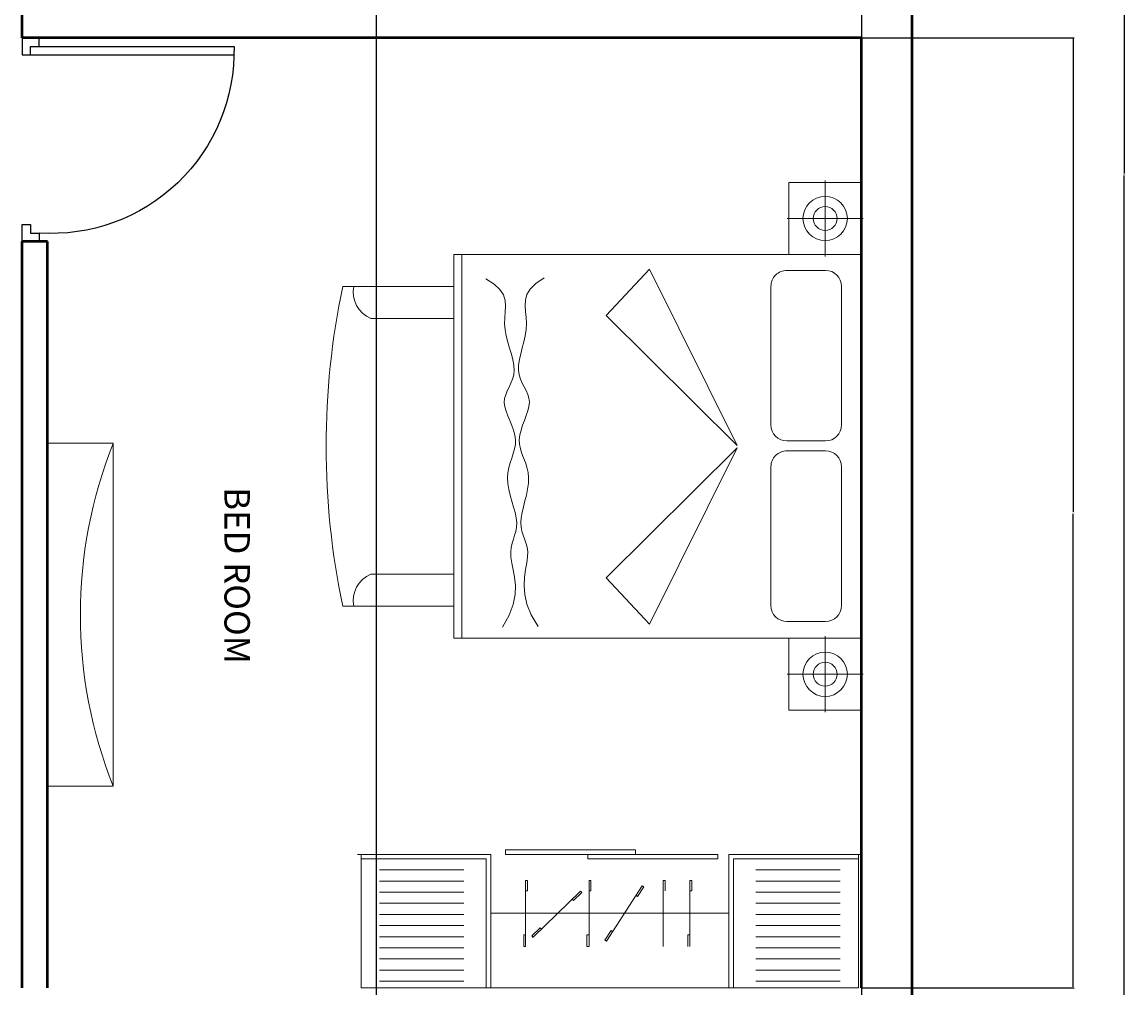
# Model space of a CAD drawing. Units: inches. Extents: x 1865 to 2541, y 1997 to 2759.
# Tile 5 of 11: x 2346 to 2541, y 2234 to 2405. Entities that reach past the tile are written whole.
import ezdxf

# ---------------------------------------------------------------- set-up
doc = ezdxf.new("R2010")
doc.units = ezdxf.units.IN
for name, color, linetype, lineweight in [('A-ANNO-DIMS', 2, 'Continuous', 18), ('A-AREA-IDEN', 4, 'Continuous', 18), ('A-WALL', 7, 'Continuous', 50), ('BED', 42, 'Continuous', 13), ('CUPBOARD', 61, 'Continuous', 18), ('DOOR', 1, 'Continuous', 25), ('TV', 3, 'Continuous', 18)]:
    doc.layers.add(name, color=color, linetype=linetype, lineweight=lineweight)
doc.styles.get("Standard").update_dxf_attribs({"font": 'arial.ttf'})
doc.dimstyles.get("Standard").update_dxf_attribs({"dimtxt": 0.18, "dimasz": 0.18, "dimexe": 0.18, "dimexo": 0.0625, "dimgap": 0.09, "dimtad": 0, "dimtih": 1, "dimtoh": 1, "dimdec": 4, "dimzin": 0, "dimdsep": 46, "dimtxsty": 'Standard', "dimcen": 0.09, "dimadec": 0, "dimazin": 0, "dimtfac": 1, "dimtdec": 4, "dimtofl": 0, "dimtmove": 0, "dimatfit": 3, "dimfxl": 1, "dimtolj": 1, "dimtzin": 0, "dimarcsym": 0})

# ---------------------------------------------------------------- blocks, each defined once
blk = doc.blocks.new('A$C34930FF8')
at = {"ltscale": 0.05}
for p, q in [((0, 2252.4), (0, 16.8)), ((600, 2252.4), (0, 2252.4)), ((185.4, 1513), (185.4, 1521.5)), ((237.7, 1513), (237.7, 1521.5)), ((436.7, 1513), (436.7, 1504.4)), ((482.5, 1513), (482.5, 1504.4)), ((227.1, 1479.2), (233.2, 1485.2)), ((263.6, 1441.7), (269.7, 1447.7)), ((398.2, 1303.6), (392.1, 1297.6)), ((434.8, 1266.1), (428.7, 1260.1)), ((185.4, 1229.1), (185.4, 1237.7)), ((237.7, 1229.1), (237.7, 1237.7)), ((436.7, 1228.2), (436.7, 1219.7)), ((482.5, 1228.2), (482.5, 1219.7)), ((209.5, 1150.1), (214.1, 1157.3)), ((253.5, 1121.8), (258.1, 1129)), ((415.3, 1017.6), (410.6, 1010.5)), ((459.3, 989.3), (454.7, 982.1)), ((482.5, 894.9), (482.5, 886.3)), ((237.7, 775.3), (237.7, 783.9)), ((436.7, 775.3), (436.7, 766.8)), ((482.5, 775.3), (482.5, 766.8)), ((600, 16.8), (0, 16.8))]:
    blk.add_line(p, q, dxfattribs=at)
for p, q in [((580, 1690.9), (580, 2252.4)), ((600, 1669.3), (600, 2269.3)), ((30, 1790.9), (30, 2169.3)), ((80, 1790.9), (80, 2169.3)), ((130, 1790.9), (130, 2169.3)), ((180, 1790.9), (180, 2169.3)), ((230, 1790.9), (230, 2169.3)), ((280, 1790.9), (280, 2169.3)), ((330, 1790.9), (330, 2169.3)), ((380, 1790.9), (380, 2169.3)), ((430, 1790.9), (430, 2169.3)), ((480, 1790.9), (480, 2169.3)), ((530, 1790.9), (530, 2169.3)), ((580, 1690.9), (0, 1690.9)), ((600, 1669.3), (0, 1669.3)), ((335.4, 1666.1), (335.4, 603.1)), ((600, 1603.3), (620, 1603.3)), ((600, 1018.7), (600, 1603.3)), ((620, 1603.3), (620, 1018.7)), ((237.7, 1521.5), (185.4, 1521.5)), ((482.5, 1513), (185.4, 1513)), ((436.7, 1504.4), (482.5, 1504.4)), ((434.8, 1266.1), (227.4, 1478.9)), ((269.7, 1447.7), (233.2, 1485.2)), ((428.7, 1260.1), (392.1, 1297.6)), ((237.7, 1237.7), (185.4, 1237.7)), ((482.5, 1228.2), (185.4, 1228.2)), ((436.7, 1219.7), (482.5, 1219.7)), ((600, 1233.4), (580, 1233.4)), ((580, 1233.4), (580, 648.7)), ((600, 648.7), (600, 1233.4)), ((459.3, 989.3), (209.5, 1150.1)), ((258.1, 1129), (214.1, 1157.3)), ((454.7, 982.1), (410.6, 1010.5)), ((620, 1018.7), (600, 1018.7)), ((482.5, 894.9), (185.4, 894.9)), ((436.7, 886.3), (482.5, 886.3)), ((237.7, 783.9), (185.4, 783.9)), ((482.5, 775.3), (185.4, 775.3)), ((436.7, 766.8), (482.5, 766.8)), ((580, 648.7), (600, 648.7)), ((600, 600), (0, 600)), ((600, 600), (600, 0)), ((580, 578.3), (0, 578.3)), ((580, 578.3), (580, 16.8)), ((30, 478.3), (30, 100)), ((80, 478.3), (80, 100)), ((130, 478.3), (130, 100)), ((180, 478.3), (180, 100)), ((230, 478.3), (230, 100)), ((280, 478.3), (280, 100)), ((330, 478.3), (330, 100)), ((380, 478.3), (380, 100)), ((430, 478.3), (430, 100)), ((480, 478.3), (480, 100)), ((530, 478.3), (530, 100))]:
    blk.add_line(p, q)
blk = doc.blocks.new('A$C4F543DC7')
for p, q in [((0.0134, 3.35, -0.1688), (3.3134, 3.35, -0.1688)), ((0.4634, 3.35, -0.1688), (0.0134, 3.35, -0.1688)), ((0.0134, 2.896, -0.1688), (0.0134, 3.35, -0.1688)), ((0.0134, 3.35, -0.1688), (0.0134, 2.896, -0.1688)), ((0.2381, 3.1233, -0.4388), (0.2381, 3.3614, -0.4388)), ((0.4634, 3.35, -0.1688), (0.4634, 0.8, -0.1688)), ((2.8634, 3.35, -0.1688), (0.4634, 3.35, -0.1688)), ((0.4634, 2.896, -0.1688), (0.4634, 3.35, -0.1688)), ((2.8634, 0.8, -0.1688), (2.8634, 3.35, -0.1688)), ((2.8634, 3.35, -0.1688), (3.3134, 3.35, -0.1688)), ((2.8634, 2.896, -0.1688), (2.8634, 3.35, -0.1688)), ((3.0888, 3.1233, -0.4388), (3.0888, 3.3614, -0.4388)), ((3.3134, 3.35, -0.1688), (3.3134, 2.896, -0.1688)), ((3.3134, 3.35, -0.1688), (3.3134, 2.896, -0.1688)), ((1.5354, 3.226, -0.1688), (0.6684, 3.226, -0.1688)), ((2.6644, 3.226, -0.1688), (1.7974, 3.226, -0.1688)), ((0.2381, 3.1233, -0.4388), (0, 3.1233, -0.4388)), ((0.2381, 3.1233, -0.4388), (0.4762, 3.1233, -0.4388)), ((0.2381, 3.1233, -0.4388), (0.2381, 2.8852, -0.4388)), ((0.5684, 3.126, -0.1688), (0.5684, 2.884, -0.1688)), ((1.6354, 2.884, -0.1688), (1.6354, 3.126, -0.1688)), ((1.6974, 3.126, -0.1688), (1.6974, 2.884, -0.1688)), ((2.7644, 2.884, -0.1688), (2.7644, 3.126, -0.1688)), ((3.0888, 3.1233, -0.4388), (2.8507, 3.1233, -0.4388)), ((3.0888, 3.1233, -0.4388), (3.0888, 2.8852, -0.4388)), ((3.0888, 3.1233, -0.4388), (3.3269, 3.1233, -0.4388)), ((0.4634, 2.896, -0.1688), (0.0134, 2.896, -0.1688)), ((0.0134, 2.896, -0.1688), (0.4634, 2.896, -0.1688)), ((0.4634, 0.8, -0.1688), (0.4634, 2.896, -0.1688)), ((2.8634, 2.896, -0.1688), (2.8634, 0.8, -0.1688)), ((3.3134, 2.896, -0.1688), (2.8634, 2.896, -0.1688)), ((3.3134, 2.896, -0.1688), (2.8634, 2.896, -0.1688)), ((0.6684, 2.784, -0.1688), (1.5354, 2.784, -0.1688)), ((1.7974, 2.784, -0.1688), (2.6644, 2.784, -0.1688)), ((1.6534, 2.573, -0.1688), (0.5504, 2.025, -0.1688)), ((0.8414, 1.752, -0.1688), (1.6534, 2.573, -0.1688)), ((2.4814, 1.752, -0.1688), (1.6694, 2.573, -0.1688)), ((1.6694, 2.573, -0.1688), (2.7724, 2.025, -0.1688)), ((0.5504, 2.025, -0.1688), (0.8414, 1.752, -0.1688)), ((2.7724, 2.025, -0.1688), (2.4814, 1.752, -0.1688)), ((0.5369, 1.3267, -0.1688), (0.6088, 1.2835, -0.1688)), ((2.683, 1.312, -0.1688), (2.7182, 1.3641, -0.1688)), ((0.6088, 1.2835, -0.1688), (0.6756, 1.2566, -0.1688)), ((0.6756, 1.2566, -0.1688), (0.7373, 1.2428, -0.1688)), ((0.8457, 1.242, -0.1688), (0.8925, 1.2489, -0.1688)), ((0.8925, 1.2489, -0.1688), (0.9345, 1.2564, -0.1688)), ((0.9345, 1.2564, -0.1688), (0.9718, 1.2615, -0.1688)), ((0.9718, 1.2615, -0.1688), (1.0044, 1.2617, -0.1688)), ((1.0044, 1.2617, -0.1688), (1.0334, 1.2578, -0.1688)), ((1.0334, 1.2578, -0.1688), (1.0597, 1.2509, -0.1688)), ((1.0597, 1.2509, -0.1688), (1.0842, 1.2424, -0.1688)), ((1.2852, 1.2347, -0.1688), (1.3218, 1.2441, -0.1688)), ((1.3218, 1.2441, -0.1688), (1.3591, 1.2533, -0.1688)), ((1.3591, 1.2533, -0.1688), (1.3963, 1.2612, -0.1688)), ((1.3963, 1.2612, -0.1688), (1.4328, 1.2664, -0.1688)), ((1.4328, 1.2664, -0.1688), (1.4679, 1.2677, -0.1688)), ((1.4679, 1.2677, -0.1688), (1.501, 1.2643, -0.1688)), ((1.501, 1.2643, -0.1688), (1.5324, 1.257, -0.1688)), ((1.5324, 1.257, -0.1688), (1.5624, 1.2473, -0.1688)), ((1.5624, 1.2473, -0.1688), (1.5915, 1.2365, -0.1688)), ((1.8258, 1.2417, -0.1688), (1.8557, 1.2531, -0.1688)), ((1.8557, 1.2531, -0.1688), (1.8849, 1.263, -0.1688)), ((1.8849, 1.263, -0.1688), (1.913, 1.2698, -0.1688)), ((1.913, 1.2698, -0.1688), (1.9397, 1.2722, -0.1688)), ((1.9397, 1.2722, -0.1688), (1.9649, 1.2692, -0.1688)), ((1.9649, 1.2692, -0.1688), (1.989, 1.2617, -0.1688)), ((1.989, 1.2617, -0.1688), (2.0124, 1.2512, -0.1688)), ((2.0124, 1.2512, -0.1688), (2.0359, 1.2391, -0.1688)), ((2.3173, 1.2378, -0.1688), (2.3558, 1.2465, -0.1688)), ((2.3558, 1.2465, -0.1688), (2.3944, 1.2527, -0.1688)), ((2.3944, 1.2527, -0.1688), (2.4325, 1.255, -0.1688)), ((2.4325, 1.255, -0.1688), (2.4698, 1.2529, -0.1688)), ((2.4698, 1.2529, -0.1688), (2.5064, 1.2488, -0.1688)), ((2.5064, 1.2488, -0.1688), (2.5423, 1.2459, -0.1688)), ((2.5423, 1.2459, -0.1688), (2.5777, 1.2476, -0.1688)), ((2.5777, 1.2476, -0.1688), (2.6129, 1.257, -0.1688)), ((2.6129, 1.257, -0.1688), (2.6479, 1.2774, -0.1688)), ((2.6479, 1.2774, -0.1688), (2.683, 1.312, -0.1688)), ((0.6743, 1.1706, -0.1688), (0.7364, 1.1825, -0.1688)), ((0.7364, 1.1825, -0.1688), (0.7931, 1.1846, -0.1688)), ((0.7373, 1.2428, -0.1688), (0.794, 1.239, -0.1688)), ((0.7931, 1.1846, -0.1688), (0.8447, 1.1799, -0.1688)), ((0.794, 1.239, -0.1688), (0.8457, 1.242, -0.1688)), ((0.8447, 1.1799, -0.1688), (0.8913, 1.1716, -0.1688)), ((1.0831, 1.172, -0.1688), (1.1072, 1.18, -0.1688)), ((1.0842, 1.2424, -0.1688), (1.1081, 1.2336, -0.1688)), ((1.1072, 1.18, -0.1688), (1.1316, 1.1872, -0.1688)), ((1.1081, 1.2336, -0.1688), (1.1322, 1.2257, -0.1688)), ((1.1316, 1.1872, -0.1688), (1.1573, 1.192, -0.1688)), ((1.1322, 1.2257, -0.1688), (1.1577, 1.2201, -0.1688)), ((1.1573, 1.192, -0.1688), (1.1851, 1.1932, -0.1688)), ((1.1577, 1.2201, -0.1688), (1.1855, 1.218, -0.1688)), ((1.1851, 1.1932, -0.1688), (1.2158, 1.1898, -0.1688)), ((1.1855, 1.218, -0.1688), (1.2163, 1.2204, -0.1688)), ((1.2158, 1.1898, -0.1688), (1.2491, 1.1828, -0.1688)), ((1.2163, 1.2204, -0.1688), (1.2498, 1.2264, -0.1688)), ((1.2491, 1.1828, -0.1688), (1.2842, 1.1734, -0.1688)), ((1.2498, 1.2264, -0.1688), (1.2852, 1.2347, -0.1688)), ((1.5915, 1.2365, -0.1688), (1.6199, 1.2259, -0.1688)), ((1.6191, 1.1716, -0.1688), (1.6475, 1.1797, -0.1688)), ((1.6199, 1.2259, -0.1688), (1.6481, 1.2169, -0.1688)), ((1.6475, 1.1797, -0.1688), (1.676, 1.1849, -0.1688)), ((1.6481, 1.2169, -0.1688), (1.6765, 1.2108, -0.1688)), ((1.676, 1.1849, -0.1688), (1.7049, 1.1858, -0.1688)), ((1.6765, 1.2108, -0.1688), (1.7053, 1.209, -0.1688)), ((1.7049, 1.1858, -0.1688), (1.7344, 1.1816, -0.1688)), ((1.7053, 1.209, -0.1688), (1.7349, 1.2124, -0.1688)), ((1.7344, 1.1816, -0.1688), (1.7643, 1.1731, -0.1688)), ((1.7349, 1.2124, -0.1688), (1.7651, 1.2199, -0.1688)), ((1.7651, 1.2199, -0.1688), (1.7955, 1.2301, -0.1688)), ((1.7955, 1.2301, -0.1688), (1.8258, 1.2417, -0.1688)), ((2.0359, 1.2391, -0.1688), (2.0599, 1.2269, -0.1688)), ((2.0599, 1.2269, -0.1688), (2.0849, 1.216, -0.1688)), ((2.0849, 1.216, -0.1688), (2.1117, 1.2077, -0.1688)), ((2.1112, 1.1743, -0.1688), (2.1403, 1.1775, -0.1688)), ((2.1117, 1.2077, -0.1688), (2.1407, 1.2037, -0.1688)), ((2.1403, 1.1775, -0.1688), (2.1718, 1.1755, -0.1688)), ((2.1407, 1.2037, -0.1688), (2.1723, 1.2047, -0.1688)), ((2.1718, 1.1755, -0.1688), (2.2056, 1.1691, -0.1688)), ((2.1723, 1.2047, -0.1688), (2.2062, 1.21, -0.1688)), ((2.2062, 1.21, -0.1688), (2.242, 1.2182, -0.1688)), ((2.242, 1.2182, -0.1688), (2.2791, 1.2279, -0.1688)), ((2.2791, 1.2279, -0.1688), (2.3173, 1.2378, -0.1688)), ((0.5334, 1.105, -0.1688), (0.6067, 1.1458, -0.1688)), ((0.6067, 1.1458, -0.1688), (0.6743, 1.1706, -0.1688)), ((0.8913, 1.1716, -0.1688), (0.9331, 1.1628, -0.1688)), ((0.9331, 1.1628, -0.1688), (0.9701, 1.1565, -0.1688)), ((0.9701, 1.1565, -0.1688), (1.0027, 1.1552, -0.1688)), ((1.0027, 1.1552, -0.1688), (1.0318, 1.1582, -0.1688)), ((1.0318, 1.1582, -0.1688), (1.0583, 1.1642, -0.1688)), ((1.0583, 1.1642, -0.1688), (1.0831, 1.172, -0.1688)), ((1.2842, 1.1734, -0.1688), (1.3206, 1.1629, -0.1688)), ((1.3206, 1.1629, -0.1688), (1.3575, 1.1524, -0.1688)), ((1.3575, 1.1524, -0.1688), (1.3945, 1.1434, -0.1688)), ((1.3945, 1.1434, -0.1688), (1.4308, 1.1371, -0.1688)), ((1.4308, 1.1371, -0.1688), (1.4658, 1.1347, -0.1688)), ((1.4658, 1.1347, -0.1688), (1.499, 1.137, -0.1688)), ((1.499, 1.137, -0.1688), (1.5306, 1.1433, -0.1688)), ((1.5306, 1.1433, -0.1688), (1.5609, 1.152, -0.1688)), ((1.5609, 1.152, -0.1688), (1.5903, 1.1619, -0.1688)), ((1.5903, 1.1619, -0.1688), (1.6191, 1.1716, -0.1688)), ((1.7643, 1.1731, -0.1688), (1.7944, 1.1619, -0.1688)), ((1.7944, 1.1619, -0.1688), (1.8244, 1.1494, -0.1688)), ((1.8244, 1.1494, -0.1688), (1.8539, 1.137, -0.1688)), ((1.8539, 1.137, -0.1688), (1.8827, 1.1263, -0.1688)), ((1.8827, 1.1263, -0.1688), (1.9106, 1.1186, -0.1688)), ((1.9106, 1.1186, -0.1688), (1.9373, 1.1153, -0.1688)), ((1.9373, 1.1153, -0.1688), (1.9625, 1.1176, -0.1688)), ((1.9625, 1.1176, -0.1688), (1.9868, 1.1243, -0.1688)), ((1.9868, 1.1243, -0.1688), (2.0106, 1.134, -0.1688)), ((2.0106, 1.134, -0.1688), (2.0344, 1.1454, -0.1688)), ((2.0344, 1.1454, -0.1688), (2.0588, 1.1568, -0.1688)), ((2.0588, 1.1568, -0.1688), (2.0842, 1.167, -0.1688)), ((2.0842, 1.167, -0.1688), (2.1112, 1.1743, -0.1688)), ((2.2056, 1.1691, -0.1688), (2.2411, 1.1598, -0.1688)), ((2.2411, 1.1598, -0.1688), (2.2779, 1.1489, -0.1688)), ((2.2779, 1.1489, -0.1688), (2.3157, 1.1379, -0.1688)), ((2.3157, 1.1379, -0.1688), (2.354, 1.1279, -0.1688)), ((2.354, 1.1279, -0.1688), (2.3923, 1.1205, -0.1688)), ((2.3923, 1.1205, -0.1688), (2.4304, 1.117, -0.1688)), ((2.4304, 1.117, -0.1688), (2.4677, 1.118, -0.1688)), ((2.4677, 1.118, -0.1688), (2.5043, 1.1209, -0.1688)), ((2.5043, 1.1209, -0.1688), (2.5403, 1.1226, -0.1688)), ((2.5403, 1.1226, -0.1688), (2.5757, 1.1199, -0.1688)), ((2.5757, 1.1199, -0.1688), (2.6106, 1.1094, -0.1688)), ((2.6106, 1.1094, -0.1688), (2.645, 1.0879, -0.1688)), ((2.645, 1.0879, -0.1688), (2.6789, 1.0522, -0.1688)), ((2.6789, 1.0522, -0.1688), (2.7124, 0.999, -0.1688)), ((0.4634, 0.85, -0.1688), (2.8634, 0.85, -0.1688)), ((0.4634, 0.8, -0.1688), (2.8634, 0.8, -0.1688)), ((0.6634, 0.8, -0.1688), (0.4634, 0.8, -0.1688)), ((0.6634, 0.8, -0.1688), (2.6634, 0.8, -0.1688)), ((0.6634, 0.104, -0.1688), (0.6634, 0.8, -0.1688)), ((0.6634, 0.104, -0.1688), (0.6634, 0.8, -0.1688)), ((0.8634, 0.281, -0.1688), (0.8634, 0.8, -0.1688)), ((2.4634, 0.8, -0.1688), (2.4634, 0.281, -0.1688)), ((2.8634, 0.8, -0.1688), (2.6634, 0.8, -0.1688)), ((2.6634, 0.8, -0.1688), (2.6634, 0.104, -0.1688)), ((2.6634, 0.8, -0.1688), (2.6634, 0.104, -0.1688))]:
    blk.add_line(p, q)
for centre, radius in [((0.2381, 3.1233, -0.4388), 0.139), ((3.0888, 3.1233, -0.4388), 0.139), ((0.2381, 3.1233, -0.4388), 0.075), ((3.0888, 3.1233, -0.4388), 0.075)]:
    blk.add_circle(centre, radius)
for centre, radius, start, end in [((0.6684, 3.126, -0.1688), 0.1, 90, 180), ((1.5354, 3.126, -0.1688), 0.1, 0, 90), ((1.7974, 3.126, -0.1688), 0.1, 90, 180), ((2.6644, 3.126, -0.1688), 0.1, 0, 90), ((0.6684, 2.884, -0.1688), 0.1, 180, 270), ((1.5354, 2.884, -0.1688), 0.1, 270, 0), ((1.7974, 2.884, -0.1688), 0.1, 180, 270), ((2.6644, 2.884, -0.1688), 0.1, 270, 0), ((0.6994, 0.3472, -0.1688), 0.1769, 258.2616, 338.03196), ((2.6275, 0.3472, -0.1688), 0.1769, 201.96804, 281.7384), ((1.6634, 4.8597, -0.1688), 4.8597, 258.12517, 281.87483), ((1.6634, 4.8597, -0.1688), 4.8597, 258.12517, 281.87483)]:
    blk.add_arc(centre, radius, start, end)
blk = doc.blocks.new('DOOR-SWING-36IN')
for p, q in [((34.51, 36), (37.51, 36)), ((34.51, 34.5), (34.51, 36)), ((37.51, 36), (37.51, 33)), ((36.01, 34.5), (0.01, 34.5)), ((36.01, 34.5), (34.51, 34.5)), ((36.01, 33), (36.01, 34.5)), ((36.01, 33), (0.01, 33)), ((37.51, 33), (36.01, 33)), ((37.51, 3), (36.01, 3)), ((36.01, 3), (36.01, 1.5)), ((37.51, 0), (37.51, 3)), ((36.01, 1.5), (34.51, 1.5)), ((34.51, 1.5), (34.51, 0)), ((34.51, 0), (37.51, 0))]:
    blk.add_line(p, q)
blk.add_arc((32.32, 33.75), 32.32, 178.6705, 273.8756)
blk = doc.blocks.new('TV-UNIT')
blk.add_lwpolyline([(0, 11.62), (60.65, 11.62), (60.65, 0), (0, 0)], close=True)
blk.add_arc((30.32, -76.26), 82.06, 68.3146, 111.6854)
blk = doc.blocks.new('*D41')
at = {"layer": 'A-ANNO-DIMS', "color": 0, "lineweight": -2, "transparency": 16777216}
for p, q in [((2503.31, 2721.45), (2540.92, 2721.45)), ((2540.74, 2721.27), (2540.74, 2378.49)), ((2540.74, 2035.35), (2540.74, 2378.13)), ((2136.19, 2035.17), (2540.92, 2035.17))]:
    blk.add_line(p, q, dxfattribs=at)
at = {"layer": 'A-ANNO-DIMS', "color": 0, "transparency": 16777216}
for points in [[(2540.71, 2721.27), (2540.77, 2721.27), (2540.74, 2721.45)], [(2540.71, 2035.35), (2540.77, 2035.35), (2540.74, 2035.17)]]:
    blk.add_solid(points, dxfattribs=at)
at = {"layer": 'Defpoints', "color": 0, "transparency": 16777216}
for p in [(2503.24, 2721.45), (2136.13, 2035.17), (2540.74, 2035.17)]:
    blk.add_point(p, dxfattribs=at)
at = {"layer": 'A-ANNO-DIMS', "color": 0, "transparency": 16777216, "insert": (2540.74, 2378.31), "char_height": 0.18, "attachment_point": 5}
blk.add_mtext('\\A1;686.3', dxfattribs=at)
blk = doc.blocks.new('*D56')
at = {"layer": 'A-ANNO-DIMS', "color": 0, "lineweight": -2, "transparency": 16777216}
for p, q in [((2494.31, 2402.45), (2531.92, 2402.45)), ((2531.74, 2402.27), (2531.74, 2318.63)), ((2531.74, 2234.63), (2531.74, 2318.27)), ((2494.31, 2234.45), (2531.92, 2234.45))]:
    blk.add_line(p, q, dxfattribs=at)
at = {"layer": 'A-ANNO-DIMS', "color": 0, "transparency": 16777216}
for points in [[(2531.71, 2402.27), (2531.77, 2402.27), (2531.74, 2402.45)], [(2531.71, 2234.63), (2531.77, 2234.63), (2531.74, 2234.45)]]:
    blk.add_solid(points, dxfattribs=at)
at = {"layer": 'Defpoints', "color": 0, "transparency": 16777216}
for p in [(2494.24, 2402.45), (2494.24, 2234.45), (2531.74, 2234.45)]:
    blk.add_point(p, dxfattribs=at)
at = {"layer": 'A-ANNO-DIMS', "color": 0, "transparency": 16777216, "insert": (2531.74, 2318.45), "char_height": 0.18, "attachment_point": 5}
blk.add_mtext('\\A1;168', dxfattribs=at)
blk = doc.blocks.new('*D64')
at = {"layer": 'A-ANNO-DIMS', "color": 0, "lineweight": -2, "transparency": 16777216}
for p, q in [((2408.38, 2406.89), (2408.38, 1997.49)), ((2494.24, 2406.89), (2494.24, 1997.49)), ((2408.56, 1997.67), (2450.92, 1997.67)), ((2494.06, 1997.67), (2451.7, 1997.67))]:
    blk.add_line(p, q, dxfattribs=at)
at = {"layer": 'A-ANNO-DIMS', "color": 0, "transparency": 16777216}
for points in [[(2408.56, 1997.7), (2408.56, 1997.64), (2408.38, 1997.67)], [(2494.06, 1997.7), (2494.06, 1997.64), (2494.24, 1997.67)]]:
    blk.add_solid(points, dxfattribs=at)
at = {"layer": 'Defpoints', "color": 0, "transparency": 16777216}
for p in [(2408.38, 2406.95), (2494.24, 2406.95), (2494.24, 1997.67)]:
    blk.add_point(p, dxfattribs=at)
at = {"layer": 'A-ANNO-DIMS', "color": 0, "transparency": 16777216, "insert": (2451.31, 1997.67), "char_height": 0.18, "attachment_point": 5}
blk.add_mtext('\\A1;85.87', dxfattribs=at)

msp = doc.modelspace()

# ---------------------------------------------------------------- linework, layer by layer
at = {"layer": 'A-WALL'}
for p, q in [((2503.243, 2061.4494), (2503.243, 2721.4494)), ((2345.743, 2402.4494), (2345.743, 2406.9494)), ((2350.243, 2402.4494), (2345.743, 2402.4494)), ((2494.243, 2402.4494), (2350.243, 2402.4494)), ((2494.243, 2234.4494), (2494.243, 2402.4494)), ((2345.743, 2234.4494), (2345.743, 2366.4494)), ((2350.243, 2366.4494), (2345.743, 2366.4494)), ((2350.243, 2234.4494), (2350.243, 2366.4494))]:
    msp.add_line(p, q, dxfattribs=at)

# ---------------------------------------------------------------- block references
at = {"layer": 'BED', "xscale": -28.27205529407425, "yscale": 28.27205529407425, "zscale": 28.27205529407425, "rotation": 270}
msp.add_blockref('A$C4F543DC7', (2399.5316, 2283.1929, 4.7709), dxfattribs=at)
at = {"layer": 'CUPBOARD', "xscale": 0.0393700787401575, "yscale": 0.0393700787401575, "zscale": 0.0393700787401575, "rotation": 89.99999999999999}
msp.add_blockref('A$C34930FF8', (2494.4069, 2234.4494), dxfattribs=at)
at = {"layer": 'DOOR', "extrusion": (0, 0, -1), "zscale": -1}
msp.add_blockref('DOOR-SWING-36IN', (-2383.252, 2366.449), dxfattribs=at)
at = {"layer": 'TV', "rotation": 89.99999999999923}
msp.add_blockref('TV-UNIT', (2361.8584, 2270.1115), dxfattribs=at)

# ---------------------------------------------------------------- texts
at = {"layer": 'A-AREA-IDEN', "insert": (2386.0474, 2322.9904), "char_height": 4.5, "attachment_point": 1, "rotation": 270}
msp.add_mtext_dynamic_manual_height_columns('BED ROOM', width=66.075761, gutter_width=12.5, heights=[0], dxfattribs=at)

# ---------------------------------------------------------------- dimensions: what is measured, and where the dimension line sits
at = {"layer": 'A-ANNO-DIMS'}
for base, p1, p2, angle, override, picture, middle in [((2540.743, 2035.1708), (2503.243, 2721.4494), (2136.13, 2035.1708), 90, {"dimdec": 1, "dimlfac": 1, "dimrnd": 0, "dimzin": 0, "dimdsep": 46, "dimlunit": 2}, '*D41', (2540.743, 2378.3101)), ((2531.743, 2234.4494), (2494.243, 2402.4494), (2494.243, 2234.4494), 270, {"dimdec": 0, "dimlfac": 1, "dimrnd": 0, "dimzin": 0, "dimdsep": 46, "dimlunit": 2}, '*D56', (2531.743, 2318.4494))]:
    dim = msp.add_linear_dim(base=base, p1=p1, p2=p2, angle=angle, dimstyle='Standard', override=override, dxfattribs=at)
    dim.commit()
    dim.dimension.update_dxf_attribs({"geometry": picture, "text_midpoint": middle})
dim = msp.add_linear_dim(base=(2494.243, 1997.6708), p1=(2408.3779, 2406.9494), p2=(2494.243, 2406.9494), dimstyle='Standard', override={"dimdec": 2, "dimlfac": 1, "dimrnd": 0, "dimzin": 0, "dimdsep": 46, "dimlunit": 2}, dxfattribs=at)
dim.commit()
dim.dimension.update_dxf_attribs({"geometry": '*D64', "text_midpoint": (2451.3105, 1997.6708)})

doc.saveas('drawing.dxf')
